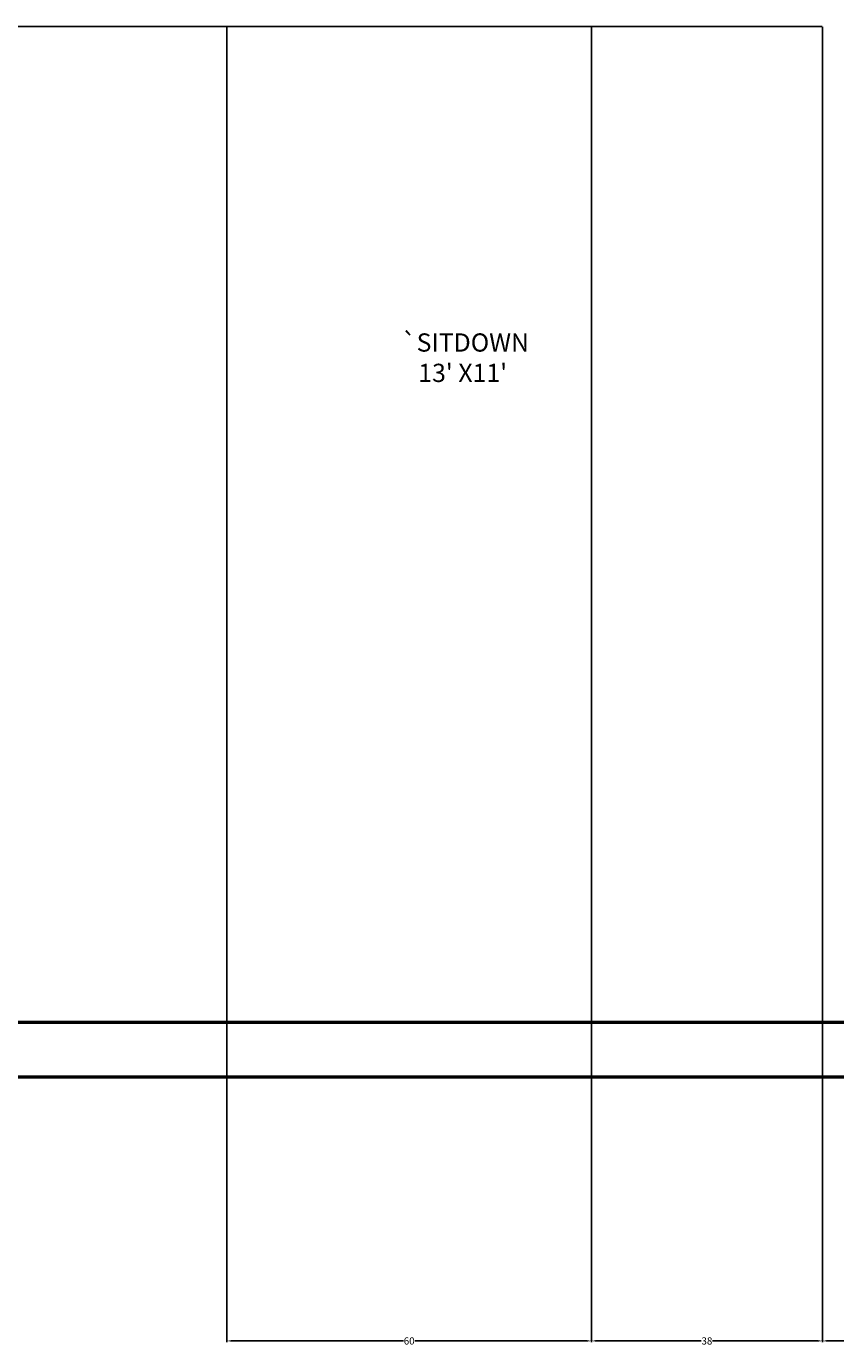
# Model space of a CAD drawing. Units: inches. Extents: x 3506 to 3958, y 1553 to 2506.
# Tile 5 of 16: x 3739 to 3872, y 1553 to 1770. Entities that reach past the tile are written whole.
import ezdxf

# ---------------------------------------------------------------- set-up
doc = ezdxf.new("R2010")
doc.units = ezdxf.units.IN
doc.header["$MEASUREMENT"] = 0
for name, color, linetype, lineweight in [('A-ANNO-DIMS', 2, 'Continuous', 18), ('A-AREA-IDEN', 7, 'Continuous', 18), ('A-WALL', 7, 'Continuous', 50)]:
    doc.layers.add(name, color=color, linetype=linetype, lineweight=lineweight)
doc.layers.add('A-WALL-PATT', color=251, linetype='Continuous', lineweight=13, true_color=0x636466)
doc.styles.get("Standard").update_dxf_attribs({"font": 'arial.ttf'})
doc.dimstyles.get("Standard").update_dxf_attribs({"dimtxt": 1.18, "dimasz": 0.68, "dimexe": 0.18, "dimexo": 0.0625, "dimgap": 0.09, "dimtad": 0, "dimtih": 1, "dimtoh": 1, "dimdec": 1, "dimzin": 0, "dimdsep": 46, "dimlunit": 3, "dimtxsty": 'Standard', "dimcen": 0.09, "dimadec": 0, "dimazin": 0, "dimtfac": 1, "dimtdec": 1, "dimtofl": 0, "dimtmove": 0, "dimatfit": 3, "dimfxl": 1, "dimtolj": 1, "dimtzin": 0, "dimarcsym": 0})

# ---------------------------------------------------------------- blocks, each defined once
blk = doc.blocks.new('*D40')
at = {"layer": 'A-ANNO-DIMS', "color": 0, "lineweight": -2, "transparency": 16777216}
for p, q in [((3869.73, 1770.33), (3869.73, 1553.76)), ((3911.73, 1597.33), (3911.73, 1553.76)), ((3870.41, 1553.94), (3889.78, 1553.94)), ((3911.05, 1553.94), (3891.68, 1553.94))]:
    blk.add_line(p, q, dxfattribs=at)
at = {"layer": 'A-ANNO-DIMS', "color": 0, "transparency": 16777216}
for points in [[(3870.41, 1554.06), (3870.41, 1553.83), (3869.73, 1553.94)], [(3911.05, 1554.06), (3911.05, 1553.83), (3911.73, 1553.94)]]:
    blk.add_solid(points, dxfattribs=at)
at = {"layer": 'Defpoints', "color": 0, "transparency": 16777216}
for p in [(3869.73, 1770.39), (3911.73, 1597.39), (3911.73, 1553.94)]:
    blk.add_point(p, dxfattribs=at)
at = {"layer": 'A-ANNO-DIMS', "color": 0, "transparency": 16777216, "insert": (3890.73, 1553.94), "char_height": 1.18, "attachment_point": 5}
blk.add_mtext('\\A1;42', dxfattribs=at)
blk = doc.blocks.new('*D63')
at = {"layer": 'A-ANNO-DIMS', "color": 0, "lineweight": -2, "transparency": 16777216}
for p, q in [((3869.67, 1800.46), (3508.1, 1800.46)), ((3508.28, 1799.78), (3508.28, 1786.12)), ((3508.28, 1771.07), (3508.28, 1784.74)), ((3869.67, 1770.39), (3508.1, 1770.39))]:
    blk.add_line(p, q, dxfattribs=at)
at = {"layer": 'A-ANNO-DIMS', "color": 0, "transparency": 16777216}
for points in [[(3508.17, 1799.78), (3508.39, 1799.78), (3508.28, 1800.46)], [(3508.17, 1771.07), (3508.39, 1771.07), (3508.28, 1770.39)]]:
    blk.add_solid(points, dxfattribs=at)
at = {"layer": 'Defpoints', "color": 0, "transparency": 16777216}
for p in [(3869.73, 1800.46), (3508.28, 1770.39), (3869.73, 1770.39)]:
    blk.add_point(p, dxfattribs=at)
at = {"layer": 'A-ANNO-DIMS', "color": 0, "transparency": 16777216, "insert": (3508.28, 1785.43), "char_height": 1.18, "attachment_point": 5}
blk.add_mtext('\\A1;30.07', dxfattribs=at)
blk = doc.blocks.new('*D64')
at = {"layer": 'A-ANNO-DIMS', "color": 0, "lineweight": -2, "transparency": 16777216}
for p, q in [((3771.73, 1770.33), (3771.73, 1553.76)), ((3831.73, 1770.33), (3831.73, 1553.76)), ((3772.41, 1553.94), (3800.79, 1553.94)), ((3831.05, 1553.94), (3802.67, 1553.94))]:
    blk.add_line(p, q, dxfattribs=at)
at = {"layer": 'A-ANNO-DIMS', "color": 0, "transparency": 16777216}
for points in [[(3772.41, 1554.06), (3772.41, 1553.83), (3771.73, 1553.94)], [(3831.05, 1554.06), (3831.05, 1553.83), (3831.73, 1553.94)]]:
    blk.add_solid(points, dxfattribs=at)
at = {"layer": 'Defpoints', "color": 0, "transparency": 16777216}
for p in [(3771.73, 1770.39), (3831.73, 1770.39), (3831.73, 1553.94)]:
    blk.add_point(p, dxfattribs=at)
at = {"layer": 'A-ANNO-DIMS', "color": 0, "transparency": 16777216, "insert": (3801.73, 1553.94), "char_height": 1.18, "attachment_point": 5}
blk.add_mtext('\\A1;60', dxfattribs=at)
blk = doc.blocks.new('*D65')
at = {"layer": 'A-ANNO-DIMS', "color": 0, "lineweight": -2, "transparency": 16777216}
for p, q in [((3831.73, 1770.33), (3831.73, 1553.76)), ((3869.73, 1770.33), (3869.73, 1553.76)), ((3832.41, 1553.94), (3849.79, 1553.94)), ((3869.05, 1553.94), (3851.67, 1553.94))]:
    blk.add_line(p, q, dxfattribs=at)
at = {"layer": 'A-ANNO-DIMS', "color": 0, "transparency": 16777216}
for points in [[(3832.41, 1554.06), (3832.41, 1553.83), (3831.73, 1553.94)], [(3869.05, 1554.06), (3869.05, 1553.83), (3869.73, 1553.94)]]:
    blk.add_solid(points, dxfattribs=at)
at = {"layer": 'Defpoints', "color": 0, "transparency": 16777216}
for p in [(3831.73, 1770.39), (3869.73, 1770.39), (3869.73, 1553.94)]:
    blk.add_point(p, dxfattribs=at)
at = {"layer": 'A-ANNO-DIMS', "color": 0, "transparency": 16777216, "insert": (3850.73, 1553.94), "char_height": 1.18, "attachment_point": 5}
blk.add_mtext('\\A1;38', dxfattribs=at)

msp = doc.modelspace()

# ---------------------------------------------------------------- hatches: boundary and pattern name
at = {"layer": 'A-WALL-PATT'}
h = msp.add_hatch(dxfattribs=at)
h.set_pattern_fill('ANSI31', color=256)
h.paths.add_polyline_path([(3911.7302, 2461.3942), (3551.7302, 2461.3942), (3551.7302, 2152.516), (3560.7302, 2152.516), (3560.7302, 2116.516), (3551.7302, 2116.516), (3551.7302, 1920.5711), (3556.2302, 1920.5711), (3560.7302, 1920.5711), (3560.7302, 2000.3942), (3692.7302, 2000.3942), (3692.7302, 1997.3942), (3697.7302, 1997.3942), (3697.7302, 2000.3942), (3771.7302, 2000.3942), (3771.7302, 1997.3942), (3776.7302, 1997.3942), (3776.7302, 1997.7206), (3778.5802, 1997.7206), (3807.5802, 1997.7206), (3807.5802, 1996.4519), (3778.5802, 1996.4519), (3778.5802, 1997.7206), (3776.7302, 1997.7206), (3776.7302, 1997.3942), (3771.7302, 1997.3942), (3771.7302, 2000.3942), (3697.7302, 2000.3942), (3697.7302, 1997.3942), (3692.7302, 1997.3942), (3689.8302, 1997.3942), (3689.8302, 1995.8192), (3653.8302, 1995.8192), (3653.8302, 1997.3942), (3689.8302, 1997.3942), (3692.7302, 1997.3942), (3692.7302, 2000.3942), (3560.7302, 2000.3942), (3560.7302, 1920.5711), (3551.7302, 1920.5711), (3551.7302, 1884.5711), (3551.7302, 1597.3942), (3911.7302, 1597.3942)], flags=17)
h.paths.add_polyline_path([(3596.7302, 2005.3942), (3596.7302, 2057.3035, -0.38730371), (3569.1778, 2085), (3569.15, 2085), (3569.15, 2086.2688), (3598.15, 2086.2688), (3598.15, 2085), (3569.1778, 2085, 0.38730371), (3596.7302, 2057.3035), (3596.7302, 2057.3942), (3601.7302, 2057.3942), (3601.7302, 2055.3942), (3630.7302, 2055.3942), (3630.7302, 2034.3942), (3694.7302, 2034.3942), (3694.7302, 2053.3942), (3699.7302, 2053.3942), (3699.7302, 2005.3942), (3860.7302, 2005.3942), (3860.7302, 2173.3942), (3771.7302, 2173.3942), (3771.7302, 2194.3942), (3776.7302, 2194.3942), (3776.7302, 2178.3942), (3860.7302, 2178.3942), (3860.7302, 2231.3942), (3601.7302, 2231.3942), (3601.7302, 2241.426), (3596.7302, 2241.426), (3596.7302, 2231.3942), (3560.7302, 2231.3942), (3560.7302, 2315.3942), (3596.7302, 2315.3942), (3596.7302, 2312.3942), (3601.7302, 2312.3942), (3601.7302, 2315.3942), (3697.7302, 2315.3942), (3697.7302, 2413.3942), (3692.7302, 2413.3942), (3692.7302, 2320.3942), (3560.7302, 2320.3942), (3560.7302, 2452.3942), (3692.7302, 2452.3942), (3692.7302, 2449.3942), (3697.7302, 2449.3942), (3697.7302, 2452.3942), (3771.7302, 2452.3942), (3771.7302, 2449.3942), (3776.7302, 2449.3942), (3776.7302, 2452.3942), (3860.7302, 2452.3942), (3860.7302, 2437.2075), (3865.2302, 2437.2075), (3865.2302, 2413.2075), (3860.7302, 2413.2075), (3860.7302, 2367.6976), (3865.2302, 2367.6976), (3869.7302, 2367.6976), (3869.7302, 2319.6976), (3860.7302, 2319.6976), (3860.7302, 2211.6248), (3869.7302, 2211.6248), (3869.7302, 2187.6248), (3860.7302, 2187.6248), (3860.7302, 2138.4346), (3865.2302, 2138.4346), (3869.7302, 2138.4346), (3869.7302, 2090.4346), (3860.7302, 2090.4346), (3860.7302, 1985.8449), (3869.7302, 1985.8449), (3869.7302, 1961.8449), (3860.7302, 1961.8449), (3860.7302, 1897.0756), (3865.2302, 1897.0756), (3869.7302, 1897.0756), (3869.7302, 1849.0756), (3860.7302, 1849.0756), (3860.7302, 1847.8112), (3860.7302, 1779.3942), (3596.7302, 1779.3942), (3596.7302, 1831.3942), (3601.7302, 1831.3942), (3601.7302, 1828.3942), (3630.7302, 1828.3942), (3630.7302, 1808.3942), (3691.7302, 1808.3942), (3691.7302, 1815.3942), (3696.7302, 1815.3942), (3696.7302, 1779.3942), (3860.7302, 1779.3942), (3860.7302, 1947.3942), (3771.7302, 1947.3942), (3771.7302, 1968.3942), (3776.7302, 1968.3942), (3776.7302, 1952.3942), (3860.7302, 1952.3942), (3860.7302, 2005.3942)], flags=0)
h.paths.add_polyline_path([(3596.7302, 2038.8546), (3601.7302, 2038.8546), (3601.7302, 2014.8546), (3596.7302, 2014.8546)], flags=0)
h.paths.add_polyline_path([(3564.1688, 2107), (3564.1688, 2167), (3644.1688, 2167), (3644.1688, 2107)], flags=0)
h.paths.add_polyline_path([(3607.0972, 2052.0208), (3620.8472, 2052.0208, -0.41421356), (3621.9931, 2050.875), (3621.9931, 2025.6667, -0.41421356), (3620.8472, 2024.5208), (3607.0972, 2024.5208, -0.41421356), (3605.9514, 2025.6667), (3605.9514, 2050.875, -0.41421356)], flags=0)
h.paths.add_polyline_path([(3578.5688, 2115), (3565.3688, 2115), (3565.3688, 2135.8), (3578.5688, 2135.8), (3578.5688, 2138.2), (3565.3688, 2138.2), (3565.3688, 2159), (3580.5688, 2159), (3580.5688, 2153.8), (3593.7688, 2167), (3593.7688, 2151.8), (3578.5688, 2151.8)], flags=0)
h.paths.add_polyline_path([(3610.9167, 2050.875), (3620.0833, 2050.875, -0.41421356), (3620.8472, 2050.1111), (3620.8472, 2039.6076, -0.41421356), (3620.0833, 2038.8438), (3610.9167, 2038.8438, -0.41421356), (3610.1528, 2039.6076), (3610.1528, 2050.1111, -0.41421356)], flags=0)
h.paths.add_polyline_path([(3610.9167, 2037.6979), (3620.0833, 2037.6979, -0.41421356), (3620.8472, 2036.934), (3620.8472, 2026.4306, -0.41421356), (3620.0833, 2025.6667), (3610.9167, 2025.6667, -0.41421356), (3610.1528, 2026.4306), (3610.1528, 2036.934, -0.41421356)], flags=0)
h.paths.add_polyline_path([(3616.2639, 2044.7639, -1), (3614.7361, 2044.7639, -1)], flags=0)
h.paths.add_polyline_path([(3615.8819, 2044.7639, -1), (3615.1181, 2044.7639, -1)], flags=0)
h.paths.add_polyline_path([(3616.2639, 2031.7778, -1), (3614.7361, 2031.7778, -1)], flags=0)
h.paths.add_polyline_path([(3615.8819, 2031.7778, -1), (3615.1181, 2031.7778, -1)], flags=0)
h.paths.add_polyline_path([(3609.7539, 2021.7868), (3626.9586, 2021.7868), (3626.9586, 2008.8833), (3609.7539, 2008.8833)], flags=0)
h.paths.add_polyline_path([(3610.4708, 2021.07), (3621.2237, 2021.07), (3621.2237, 2009.6002), (3610.4708, 2009.6002)], flags=0)
h.paths.add_polyline_path([(3611.5461, 2019.9947), (3620.1484, 2019.9947), (3620.1484, 2010.6755), (3611.5461, 2010.6755)], flags=0)
h.paths.add_polyline_path([(3621.9405, 2021.07), (3626.2417, 2021.07), (3626.2417, 2009.6002), (3621.9405, 2009.6002)], flags=0)
h.paths.add_polyline_path([(3622.6574, 2020.3531), (3625.5248, 2020.3531), (3625.5248, 2017.4857), (3622.6574, 2017.4857)], flags=0)
h.paths.add_polyline_path([(3622.6574, 2016.7688), (3625.5248, 2016.7688), (3625.5248, 2010.317), (3622.6574, 2010.317)], flags=0)
h.paths.add_polyline_path([(3624.808, 2016.0519), (3624.808, 2013.9013), (3624.0911, 2013.9013), (3624.0911, 2013.1845), (3623.3743, 2013.1845), (3623.3743, 2013.9013), (3623.3743, 2016.0519)], flags=0)
h.paths.add_polyline_path([(3623.0158, 2012.8261), (3625.1664, 2012.8261), (3625.1664, 2012.1092), (3623.0158, 2012.1092)], flags=0)
h.paths.add_polyline_path([(3623.0158, 2011.7508), (3625.1664, 2011.7508), (3625.1664, 2011.0339), (3623.0158, 2011.0339)], flags=0)
h.paths.add_polyline_path([(3650.0591, 2031.8202), (3674.0368, 2031.8202), (3674.0368, 2012.638), (3669.2413, 2012.638), (3669.2413, 2011.8388), (3672.4383, 2011.8388), (3672.4383, 2011.0395), (3651.6576, 2011.0395), (3651.6576, 2011.8388), (3654.8546, 2011.8388), (3654.8546, 2012.638), (3650.0591, 2012.638)], flags=0)
h.paths.add_polyline_path([(3658.0517, 2024.6269, -1), (3651.6576, 2024.6269, -1)], flags=0)
h.paths.add_polyline_path([(3657.2524, 2024.6269, -1), (3652.4569, 2024.6269, -1)], flags=0)
h.paths.add_polyline_path([(3656.4532, 2024.6269, -1), (3653.2561, 2024.6269, -1)], flags=0)
h.paths.add_polyline_path([(3655.6539, 2024.6269, -1), (3654.0554, 2024.6269, -1)], flags=0)
h.paths.add_polyline_path([(3657.2524, 2017.4336, -1), (3652.4569, 2017.4336, -1)], flags=0)
h.paths.add_polyline_path([(3656.4532, 2017.4336, -1), (3653.2561, 2017.4336, -1)], flags=0)
h.paths.add_polyline_path([(3655.6539, 2017.4336, -1), (3654.0554, 2017.4336, -1)], flags=0)
h.paths.add_polyline_path([(3659.6502, 2027.8239), (3664.4457, 2027.8239), (3664.4457, 2015.0358), (3659.6502, 2015.0358)], flags=0)
h.paths.add_polyline_path([(3663.6465, 2027.0247), (3663.6465, 2015.8351), (3660.4494, 2015.8351), (3660.4494, 2027.0247)], flags=0)
h.paths.add_polyline_path([(3562.6688, 1945.5), (3642.6688, 1945.5), (3642.6688, 1885.5), (3562.6688, 1885.5)], flags=0)
h.paths.add_polyline_path([(3671.6391, 2024.6269, -1), (3666.8435, 2024.6269, -1)], flags=0)
h.paths.add_polyline_path([(3670.8398, 2024.6269, -1), (3667.6428, 2024.6269, -1)], flags=0)
h.paths.add_polyline_path([(3672.4383, 2017.4336, -1), (3666.0443, 2017.4336, -1)], flags=0)
h.paths.add_polyline_path([(3670.0405, 2024.6269, -1), (3668.442, 2024.6269, -1)], flags=0)
h.paths.add_polyline_path([(3671.6391, 2017.4336, -1), (3666.8435, 2017.4336, -1)], flags=0)
h.paths.add_polyline_path([(3670.8398, 2017.4336, -1), (3667.6428, 2017.4336, -1)], flags=0)
h.paths.add_polyline_path([(3592.2688, 1945.5), (3592.2688, 1930.3), (3577.0688, 1930.3), (3577.0688, 1893.5), (3563.8688, 1893.5), (3563.8688, 1914.3), (3577.0688, 1914.3), (3577.0688, 1916.7), (3563.8688, 1916.7), (3563.8688, 1937.5), (3579.0688, 1937.5), (3579.0688, 1932.3)], flags=0)
h.paths.add_polyline_path([(3670.0405, 2017.4336, -1), (3668.442, 2017.4336, -1)], flags=0)
h.paths.add_polyline_path([(3596.7302, 2283.3942), (3601.7302, 2283.3942), (3601.7302, 2265.426), (3599.2302, 2265.426), (3599.2302, 2241.426), (3596.7302, 2241.426), (3596.7302, 2265.426)], flags=0)
h.paths.add_polyline_path([(3596.7302, 1810.7006), (3601.7302, 1810.7006), (3601.7302, 1786.7006), (3596.7302, 1786.7006)], flags=0)
h.paths.add_polyline_path([(3560.7302, 1770.3942), (3738.7302, 1770.3942), (3738.7302, 1746.3942), (3738.7302, 1722.3942), (3748.7302, 1722.3942), (3748.7302, 1674.3942), (3560.7302, 1674.3942)], flags=0)
h.paths.add_polyline_path([(3728.7302, 1746.3942), (3728.7302, 1756.0642), (3738.7302, 1746.3942), (3728.7302, 1738.1582), (3728.7302, 1698.3942), (3591.2519, 1698.3942), (3591.2519, 1746.3942)], flags=0)
h.paths.add_polyline_path([(3771.7302, 2399.3942), (3771.7302, 2420.3942), (3776.7302, 2420.3942), (3776.7302, 2404.3942), (3776.7302, 2399.3942)], flags=0)
h.paths.add_polyline_path([(3911.7302, 2461.3942), (3551.7302, 2461.3942), (3551.7302, 2152.516), (3560.7302, 2152.516), (3560.7302, 2116.516), (3551.7302, 2116.516), (3551.7302, 1920.5711), (3560.7302, 1920.5711), (3560.7302, 2000.3942), (3692.7302, 2000.3942), (3692.7302, 1997.3942), (3697.7302, 1997.3942), (3697.7302, 2000.3942), (3771.7302, 2000.3942), (3771.7302, 1997.3942), (3776.7302, 1997.3942), (3776.7302, 1997.7206), (3778.5802, 1997.7206), (3807.5802, 1997.7206), (3807.5802, 1996.4519), (3778.5802, 1996.4519), (3778.5802, 1997.7206), (3776.7302, 1997.7206), (3776.7302, 1997.3942), (3771.7302, 1997.3942), (3771.7302, 2000.3942), (3697.7302, 2000.3942), (3697.7302, 1997.3942), (3692.7302, 1997.3942), (3689.8302, 1997.3942), (3689.8302, 1995.8192), (3653.8302, 1995.8192), (3653.8302, 1997.3942), (3689.8302, 1997.3942), (3692.7302, 1997.3942), (3692.7302, 2000.3942), (3560.7302, 2000.3942), (3560.7302, 1920.5711), (3551.7302, 1920.5711), (3551.7302, 1597.3942), (3911.7302, 1597.3942)], flags=17)

# ---------------------------------------------------------------- linework, layer by layer
at = {"layer": 'A-WALL'}
msp.add_line((3902.7302, 1606.3942), (3560.7302, 1606.3942), dxfattribs=at)
msp.add_lwpolyline([(3551.7302, 2461.3942), (3911.7302, 2461.3942), (3911.7302, 1597.3942), (3551.7302, 1597.3942)], close=True, dxfattribs=at)

# ---------------------------------------------------------------- texts
at = {"layer": 'A-AREA-IDEN', "insert": (3800.4762, 1719.842), "char_height": 3, "attachment_point": 1}
msp.add_mtext_dynamic_manual_height_columns("`SITDOWN\\P   13' X11'", width=46.119714, gutter_width=1, heights=[0], dxfattribs=at)

# ---------------------------------------------------------------- dimensions: what is measured, and where the dimension line sits
at = {"layer": 'A-ANNO-DIMS'}
dim = msp.add_linear_dim(base=(3508.2802, 1770.3942), p1=(3869.7302, 1800.4628), p2=(3869.7302, 1770.3942), angle=90, dimstyle='Standard', override={"dimdec": 2, "dimlfac": 1, "dimrnd": 0, "dimzin": 0, "dimdsep": 46, "dimlunit": 2}, dxfattribs=at)
dim.commit()
dim.dimension.update_dxf_attribs({"geometry": '*D63', "text_midpoint": (3508.2802, 1785.4285)})
for base, p1, p2, picture, middle in [((3831.7302, 1553.9442), (3771.7302, 1770.3942), (3831.7302, 1770.3942), '*D64', (3801.7302, 1553.9442)), ((3869.7302, 1553.9442), (3831.7302, 1770.3942), (3869.7302, 1770.3942), '*D65', (3850.7302, 1553.9442)), ((3911.7302, 1553.9442), (3869.7302, 1770.3942), (3911.7302, 1597.3942), '*D40', (3890.7302, 1553.9442))]:
    dim = msp.add_linear_dim(base=base, p1=p1, p2=p2, dimstyle='Standard', override={"dimdec": 0, "dimlfac": 1, "dimrnd": 0, "dimzin": 0, "dimdsep": 46, "dimlunit": 2}, dxfattribs=at)
    dim.commit()
    dim.dimension.update_dxf_attribs({"geometry": picture, "text_midpoint": middle})

doc.saveas('drawing.dxf')
